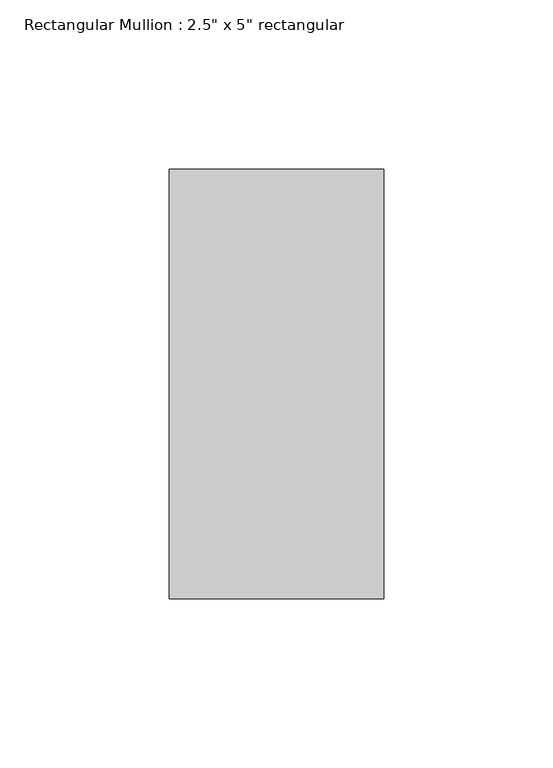
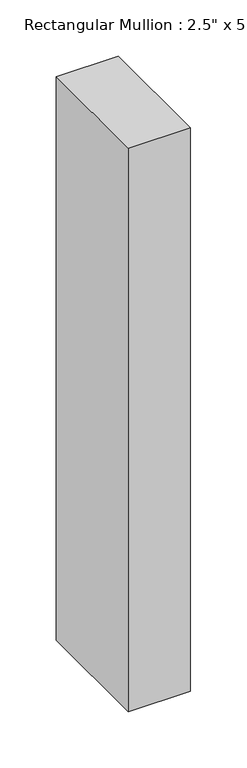
"""IFC4 building model written with IfcOpenShell, lengths in millimetres: member geometry."""

from ifc_helpers import new_model, si_unit, frame, origin, place, context, project, spatial, polyline, outline, extrude, source, transform, mapped, element, save


def member_6e77e263(model_context):
    return source(origin(), model_context, "Body", "SweptSolid", [
        extrude(outline(polyline([(31.75, 63.5), (31.75, -63.5), (-31.75, -63.5), (-31.75, 63.5), (31.75, 63.5)])), frame((0.0, 0.0, -609.6), z_axis=(0.0, 0.0, 1.0), x_axis=(1.0, 0.0, 0.0)), (0.0, 0.0, 1.0), 609.6),
    ])


if __name__ == "__main__":
    model = new_model("IFC4")
    model_context = context("Model", 3, world=origin())
    ifc_project = project(units=[si_unit("LENGTHUNIT", "METRE", prefix="MILLI")], contexts=[model_context])
    site = spatial("IfcSite", under=ifc_project)
    building = spatial("IfcBuilding", under=site)
    placement = place(None, origin())
    member_shape = member_6e77e263(model_context)
    element("IfcMember", 1, ObjectType="Rectangular Mullion : 2.5\" x 5\" rectangular", at=placement, inside=building, context=model_context, shape_type="MappedRepresentation", body=[
        mapped(member_shape, transform((0.0, 0.0, 0.0), x_axis=(1.0, 0.0, 0.0), y_axis=(0.0, 1.0, 0.0), z_axis=(0.0, 0.0, 1.0))),
    ])
    save(model, "model.ifc")

# Revit data of these elements
# Type "Rectangular Mullion : 2.5\" x 5\" rectangular"
#   built-in parameter 1007304 = 0.416667 (stored number, unit not read)
#   built-in parameter 1007301 = 0.104167 (stored number, unit not read)
#   built-in parameter 1007300 = 0.104167 (stored number, unit not read)
# Element 1 (IfcMember, "Rectangular Mullion : 2.5\" x 5\" rectangular")
#   Materials on its faces: "Iron, Ductile"
# Materials
#   "Iron, Ductile": class "Metal", colour RGB 0 0 0, transparency 0, Description = "Ductile cast iron", Cost = 0
